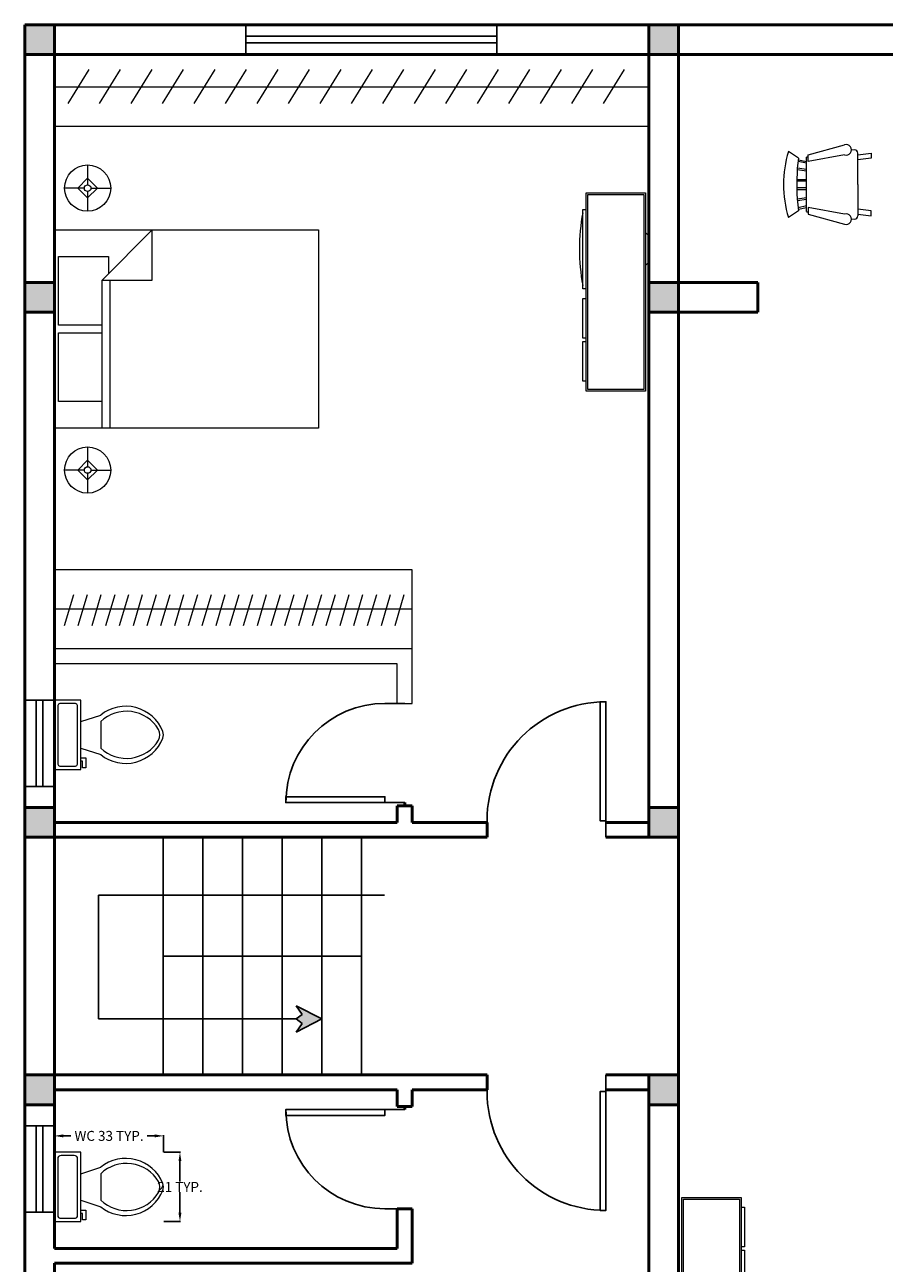
# Model space of a CAD drawing. Units: inches. Extents: x 13 to 1693, y -7 to 1519.
# Tile 2 of 10: x 116 to 377, y 360 to 735. Entities that reach past the tile are written whole.
import ezdxf

# ---------------------------------------------------------------- set-up
doc = ezdxf.new("R2010")
doc.units = ezdxf.units.IN
doc.header["$MEASUREMENT"] = 0
for name, color, linetype, lineweight in [('A-ANNO-DIMS', 2, 'Continuous', 18), ('A-DOOR', 4, 'Continuous', 25), ('A-FLOR-CASE', 5, 'Continuous', 18), ('A-FLOR-FIXT', 9, 'Continuous', 18), ('A-FLOR-STRS', 2, 'Continuous', 25), ('A-FURN', 8, 'Continuous', 18), ('A-GLAZ', 4, 'Continuous', 25), ('A-WALL', 7, 'Continuous', 50), ('A-WALL-PATT', 8, 'Continuous', 13)]:
    doc.layers.add(name, color=color, linetype=linetype, lineweight=lineweight)
doc.styles.get("Standard").update_dxf_attribs({"font": 'arial.ttf'})
doc.dimstyles.get("Standard").update_dxf_attribs({"dimtxt": 3, "dimasz": 2.68, "dimexe": 0.18, "dimexo": 0.0625, "dimgap": 0.09, "dimtad": 0, "dimtih": 1, "dimtoh": 1, "dimdec": 0, "dimzin": 0, "dimdsep": 46, "dimlunit": 3, "dimtxsty": 'Standard', "dimcen": 0.09, "dimadec": 0, "dimazin": 0, "dimtfac": 1, "dimtdec": 0, "dimtofl": 0, "dimtmove": 0, "dimatfit": 3, "dimfxl": 1, "dimtolj": 1, "dimtzin": 0, "dimarcsym": 0})

# ---------------------------------------------------------------- blocks, each defined once
blk = doc.blocks.new('*U7')
for p, q in [((0, 0), (0, -5)), ((36, 0), (36, -5))]:
    blk.add_line(p, q)
blk.add_lwpolyline([(0, 0), (0, 36), (1.75, 36), (1.75, 0)], close=True)
blk.add_arc((0, 0), 36, 0, 90)
blk = doc.blocks.new('*U8')
for p, q in [((0, 0), (0, -6)), ((30, 0), (30, -6))]:
    blk.add_line(p, q)
blk.add_lwpolyline([(0, 0), (0, 30), (1.75, 30), (1.75, 0)], close=True)
blk.add_arc((0, 0), 30, 0, 90)
blk = doc.blocks.new('Entertainment Center')
for p, q in [((-4, 0), (-5, -1)), ((4, 0), (-4, 0)), ((5, -1), (4, 0)), ((-17, -19), (-17, -1)), ((-17, -1), (43, -1)), ((-16.5, -18.5), (-16.5, -1.5)), ((-16.5, -1.5), (42.5, -1.5)), ((42.5, -1.5), (42.5, -18.5)), ((43, -1), (43, -19)), ((42.5, -18.5), (-16.5, -18.5)), ((43, -19), (-17, -19)), ((-12, -20), (-12, -19)), ((12, -20), (-12, -20)), ((12, -19), (12, -20)), ((15, -20), (15, -19)), ((27, -20), (15, -20)), ((27, -19), (27, -20)), ((28, -20), (28, -19)), ((40, -20), (28, -20)), ((40, -19), (40, -20))]:
    blk.add_line(p, q)
blk.add_arc((0, 40), 61, 259.6111, 280.3889)
blk = doc.blocks.new('Bed - Queen')
for p, q in [((0, -80.00003), (0, 0)), ((0, 0), (59.99999, 0)), ((59.99999, 0), (59.99999, -80.00003)), ((7.99999, -1.2), (28.79998, -1.2)), ((7.99999, -14.4), (7.99999, -1.2)), ((28.79998, -1.2), (28.79998, -14.4)), ((31.19999, -1.2), (51.99999, -1.2)), ((31.19999, -14.4), (31.19999, -1.2)), ((51.99999, -1.2), (51.99999, -16.4)), ((0, -14.4), (44.8, -14.4)), ((59.99999, -29.6), (44.8, -14.4)), ((44.8, -14.4), (44.8, -29.6)), ((44.8, -16.8), (0, -16.8)), ((51.99999, -16.4), (46.79936, -16.4)), ((44.8, -29.6), (59.99999, -29.6)), ((59.99999, -80.00003), (0, -80.00003))]:
    blk.add_line(p, q)
blk = doc.blocks.new('Lamp - Table')
for p, q in [((0, 7), (0, 1)), ((-1, 0), (-7, 0)), ((0, 3), (-3, 0)), ((-3, 0), (0, -3)), ((3, 0), (0, 3)), ((0, -3), (3, 0)), ((1, 0), (7, 0)), ((0, -1), (0, -7))]:
    blk.add_line(p, q)
for radius in [7, 1]:
    blk.add_circle((0, 0), radius)
blk = doc.blocks.new('Toilet - top')
for p, q in [((9.5, -6), (9.5, -2)), ((-10, -8.5), (-8, -8.5)), ((-10, -9.5), (-10, -8.5)), ((-7, -9.5), (-10, -9.5)), ((-8, -8.5), (-8, -8)), ((-7, -8), (-7, -9.5)), ((-4, -8), (-6, -14)), ((4, -8), (6, -14)), ((4, -14), (-4, -14))]:
    blk.add_line(p, q)
blk.add_lwpolyline([(10.5, -8), (10.5, 0), (-10.5, 0), (-10.5, -8)], close=True)
for points in [[(-9.5, -2), (-9.5, -6)], [(8.5, -1), (-8.5, -1)], [(-8.5, -7), (8.5, -7)]]:
    blk.add_lwpolyline(points)
for centre, radius, start, end in [((-8.62, -1.88), 0.884, 81.8699, 188.1301), ((8.62, -1.88), 0.884, 351.8699, 98.1301), ((-8.62, -6.12), 0.884, 171.8699, 278.1301), ((8.62, -6.12), 0.884, 261.8699, 8.1301), ((3.52, -21.58), 12.17, 141.4691, 247.9714), ((4.2, -21.82), 11.33, 136.3677, 238.9468), ((-3.52, -21.58), 12.17, 292.0284, 38.5307), ((-4.2, -21.82), 11.33, 301.053, 43.6321), ((0, -27.88), 4, 245.7318, 294.2682), ((0, -29), 4, 254.8605, 285.1395)]:
    blk.add_arc(centre, radius, start, end)
blk = doc.blocks.new('Chair - Rocking')
for p, q in [((-8, -4.5), (-10, -1.5)), ((8, -4.5), (10, -1.5)), ((-9, -7.5), (-12, -18.49999)), ((-7, -7.5), (-9, -7.5)), ((-9, -18.49999), (-7, -7.5)), ((-8.23428, -6.99939), (-8.3093, -7.47958)), ((-8.23041, -7), (8.23915, -7)), ((-7.5, -4.5), (-7, -7)), ((-6.5, -7), (-7.02225, -4.43)), ((-4.5, -7), (-4.96674, -4.19951)), ((-4, -7), (-4.40532, -4.16272)), ((-1.5, -4.05012), (-1.5, -7)), ((-1, -7), (-1, -4.05012)), ((1, -7), (1, -4.04655)), ((1.5, -4.05012), (1.5, -7)), ((4, -7), (4.40187, -4.18694)), ((4.5, -7), (4.96761, -4.19437)), ((6.5, -7), (7, -4.4057)), ((7.5, -4.5), (7, -7)), ((7, -7.5), (9, -7.5)), ((9, -18.49999), (7, -7.5)), ((8.31071, -7.48854), (8.23449, -7.00073)), ((9, -7.5), (12, -18.49999)), ((-10.36644, -20.64523), (-10.5, -21.49999)), ((-9, -22.49999), (-9.5, -26.49999)), ((0, -22.49999), (-9.5, -22.49999)), ((-8, -26.49999), (-7.5, -22.49999)), ((0, -22.49999), (9.5, -22.49999)), ((8, -26.49999), (7.5, -22.49999)), ((9, -22.49999), (9.5, -26.49999)), ((10.5, -21.49999), (10.3575, -20.58798)), ((-9.5, -26.49999), (-8, -26.49999)), ((9.5, -26.49999), (8, -26.49999))]:
    blk.add_line(p, q)
for centre, radius, start, end in [((0, -34.08333), 34.08333, 72.93847, 107.0615), ((0, -68.25004), 64.25, 93.92211, 97.15267), ((0, -68.25004), 64.25, 82.84733, 93.92211), ((-10.5, -18.99999), 1.58114, 161.5651, 18.43495), ((10.5, -18.99999), 1.58114, 161.5651, 18.43495), ((-9.5, -21.49999), 1, 180, 270), ((9.5, -21.49999), 1, 270, 0)]:
    blk.add_arc(centre, radius, start, end)
blk = doc.blocks.new('WIN-76')
for p, q in [((0, 9), (0, 0)), ((76.02, 9), (76.02, 0)), ((0, 5.5), (76.02, 5.5)), ((0, 3.5), (76.02, 3.5))]:
    blk.add_line(p, q)
blk = doc.blocks.new('WIN-26')
for p, q in [((9, 26.11), (0, 26.11)), ((3.5, 26.11), (3.5, 0)), ((5.5, 26.11), (5.5, 0)), ((9, 0), (0, 0))]:
    blk.add_line(p, q)
blk = doc.blocks.new('*D64')
at = {"layer": 'A-ANNO-DIMS', "color": 0, "lineweight": -2, "transparency": 16777216}
for p, q in [((125.45, 393.82), (125.45, 398.89)), ((128.13, 398.71), (130.45, 398.71)), ((155.82, 398.71), (153.5, 398.71)), ((158.5, 393.82), (158.5, 398.89))]:
    blk.add_line(p, q, dxfattribs=at)
at = {"layer": 'A-ANNO-DIMS', "color": 0, "transparency": 16777216}
for points in [[(128.13, 399.16), (128.13, 398.26), (125.45, 398.71)], [(155.82, 399.16), (155.82, 398.26), (158.5, 398.71)]]:
    blk.add_solid(points, dxfattribs=at)
at = {"layer": 'Defpoints', "color": 0, "transparency": 16777216}
for p in [(125.45, 398.71), (125.45, 393.75), (158.5, 393.75)]:
    blk.add_point(p, dxfattribs=at)
at = {"layer": 'A-ANNO-DIMS', "color": 0, "transparency": 16777216, "insert": (141.98, 398.71), "char_height": 3, "attachment_point": 5}
blk.add_mtext('\\A1;WC 33 TYP.', dxfattribs=at)
blk = doc.blocks.new('*D65')
at = {"layer": 'A-ANNO-DIMS', "color": 0, "lineweight": -2, "transparency": 16777216}
for p, q in [((158.56, 393.75), (163.64, 393.75)), ((163.46, 391.07), (163.46, 384.85)), ((163.46, 375.43), (163.46, 381.66)), ((158.56, 372.75), (163.64, 372.75))]:
    blk.add_line(p, q, dxfattribs=at)
at = {"layer": 'A-ANNO-DIMS', "color": 0, "transparency": 16777216}
for points in [[(163.01, 391.07), (163.9, 391.07), (163.46, 393.75)], [(163.01, 375.43), (163.9, 375.43), (163.46, 372.75)]]:
    blk.add_solid(points, dxfattribs=at)
at = {"layer": 'Defpoints', "color": 0, "transparency": 16777216}
for p in [(158.5, 393.75), (163.46, 393.75), (158.5, 372.75)]:
    blk.add_point(p, dxfattribs=at)
at = {"layer": 'A-ANNO-DIMS', "color": 0, "transparency": 16777216, "insert": (163.46, 383.25), "char_height": 3, "attachment_point": 5}
blk.add_mtext('\\A1;21 TYP.', dxfattribs=at)

msp = doc.modelspace()

# ---------------------------------------------------------------- hatches: boundary and pattern name
at = {"layer": 'A-WALL-PATT'}
h = msp.add_hatch(color=256, dxfattribs=at)
h.dxf.hatch_style = 1
h.paths.add_polyline_path([(125.45, 735.15), (116.45, 735.15), (116.45, 726.15), (125.45, 726.15)])
h.paths.add_polyline_path([(125.45, 657.15), (116.45, 657.15), (116.45, 648.15), (125.45, 648.15)])
h.paths.add_polyline_path([(125.45, 498.15), (116.45, 498.15), (116.45, 489.15), (125.45, 489.15)])
h.paths.add_polyline_path([(125.45, 417.15), (116.45, 417.15), (116.45, 408.15), (125.45, 408.15)])
h.paths.add_polyline_path([(125.45, 177.15), (116.45, 177.15), (116.45, 168.15), (125.45, 168.15)])
h.paths.add_polyline_path([(314.45, 177.15), (305.45, 177.15), (305.45, 168.15), (314.45, 168.15)])
h.paths.add_polyline_path([(314.45, 417.15), (305.45, 417.15), (305.45, 408.15), (314.45, 408.15)])
h.paths.add_polyline_path([(314.45, 498.15), (305.45, 498.15), (305.45, 489.15), (314.45, 489.15)])
h.paths.add_polyline_path([(314.45, 657.15), (305.45, 657.15), (305.45, 648.15), (314.45, 648.15)])
h.paths.add_polyline_path([(314.45, 735.15), (305.45, 735.15), (305.45, 726.15), (314.45, 726.15)])
h = msp.add_hatch(color=256, dxfattribs=at)
h.dxf.hatch_style = 1
h.paths.add_polyline_path([(198.64, 438.07), (200.46, 435.46), (198.61, 434.11), (200.46, 432.76), (198.64, 430.15), (206.42, 434.11)])

# ---------------------------------------------------------------- linework, layer by layer
at = {"layer": 'A-FLOR-CASE'}
for p, q in [((135.81, 721.58), (129.45, 711.36)), ((145.35, 721.58), (138.99, 711.36)), ((154.89, 721.58), (148.53, 711.36)), ((164.43, 721.58), (158.07, 711.36)), ((173.97, 721.58), (167.61, 711.36)), ((183.51, 721.58), (177.15, 711.36)), ((193.05, 721.58), (186.69, 711.36)), ((202.59, 721.58), (196.23, 711.36)), ((212.13, 721.58), (205.77, 711.36)), ((221.67, 721.58), (215.31, 711.36)), ((231.21, 721.58), (224.85, 711.36)), ((240.75, 721.58), (234.39, 711.36)), ((250.29, 721.58), (243.93, 711.36)), ((259.82, 721.58), (253.46, 711.36)), ((269.36, 721.58), (263, 711.36)), ((278.9, 721.58), (272.54, 711.36)), ((288.44, 721.58), (282.08, 711.36)), ((297.98, 721.58), (291.62, 711.36)), ((125.45, 716.33), (305.45, 716.33)), ((125.45, 704.45), (305.45, 704.45)), ((233.77, 570.15), (125.45, 570.15)), ((233.77, 546.15), (233.77, 570.15)), ((131.17, 562.5), (128.39, 553.12)), ((135.35, 562.5), (132.56, 553.12)), ((139.52, 562.5), (136.74, 553.12)), ((143.69, 562.5), (140.91, 553.12)), ((147.86, 562.5), (145.08, 553.12)), ((152.04, 562.5), (149.25, 553.12)), ((156.21, 562.5), (153.43, 553.12)), ((160.38, 562.5), (157.6, 553.12)), ((164.55, 562.5), (161.77, 553.12)), ((168.72, 562.5), (165.94, 553.12)), ((172.9, 562.5), (170.12, 553.12)), ((177.07, 562.5), (174.29, 553.12)), ((181.24, 562.5), (178.46, 553.12)), ((185.41, 562.5), (182.63, 553.12)), ((189.59, 562.5), (186.81, 553.12)), ((193.76, 562.5), (190.98, 553.12)), ((197.93, 562.5), (195.15, 553.12)), ((202.1, 562.5), (199.32, 553.12)), ((206.28, 562.5), (203.49, 553.12)), ((210.45, 562.5), (207.67, 553.12)), ((214.62, 562.5), (211.84, 553.12)), ((218.79, 562.5), (216.01, 553.12)), ((222.97, 562.5), (220.18, 553.12)), ((227.14, 562.5), (224.36, 553.12)), ((231.31, 562.5), (228.53, 553.12)), ((233.77, 558.15), (125.45, 558.15)), ((233.77, 546.15), (125.45, 546.15)), ((233.77, 529.65), (233.77, 546.15)), ((229.27, 541.65), (125.45, 541.65)), ((229.27, 529.65), (229.27, 541.65)), ((229.27, 529.65), (233.77, 529.65))]:
    msp.add_line(p, q, dxfattribs=at)
at = {"layer": 'A-FLOR-STRS'}
for p, q in [((158.42, 489.15), (158.42, 417.15)), ((170.42, 489.15), (170.42, 417.15)), ((182.42, 489.15), (182.42, 417.15)), ((194.42, 489.15), (194.42, 417.15)), ((206.42, 489.15), (206.42, 417.15)), ((218.42, 489.15), (218.42, 417.15)), ((225.37, 471.55), (138.82, 471.55)), ((138.82, 471.55), (138.82, 434.11)), ((158.42, 453.15), (218.42, 453.15)), ((200.46, 435.46), (198.61, 434.11)), ((206.42, 434.11), (198.64, 438.07)), ((198.64, 438.07), (200.46, 435.46)), ((138.82, 434.11), (198.61, 434.11)), ((200.46, 432.76), (198.61, 434.11)), ((206.42, 434.11), (198.64, 430.15)), ((198.64, 430.15), (200.46, 432.76))]:
    msp.add_line(p, q, dxfattribs=at)
at = {"layer": 'A-WALL'}
for p, q in [((116.45, 168.15), (116.45, 735.15)), ((683.45, 735.15), (116.45, 735.15)), ((125.45, 364.65), (125.45, 735.15)), ((305.45, 735.15), (305.45, 489.15)), ((314.45, 735.15), (314.45, 489.15)), ((485.45, 726.15), (116.45, 726.15)), ((125.45, 657.15), (116.45, 657.15)), ((338.45, 657.15), (305.45, 657.15)), ((338.45, 648.15), (338.45, 657.15)), ((125.45, 648.15), (116.45, 648.15)), ((338.45, 648.15), (305.45, 648.15)), ((231.52, 498.65), (231.52, 499.65)), ((229.27, 493.65), (229.27, 498.65)), ((233.77, 498.65), (229.27, 498.65)), ((233.77, 493.65), (233.77, 498.65)), ((233.77, 493.65), (233.77, 498.65)), ((229.27, 493.65), (125.45, 493.65)), ((256.45, 493.65), (233.77, 493.65)), ((256.45, 493.65), (256.45, 489.15)), ((305.45, 493.65), (292.45, 493.65)), ((256.45, 489.15), (116.45, 489.15)), ((293.45, 489.15), (292.45, 489.15)), ((314.45, 489.15), (293.45, 489.15)), ((314.45, 489.15), (314.45, 417.15)), ((256.45, 417.15), (116.45, 417.15)), ((256.45, 412.65), (256.45, 417.15)), ((293.45, 417.15), (292.45, 417.15)), ((314.45, 417.15), (293.45, 417.15)), ((305.45, 417.15), (305.45, 168.15)), ((314.45, 417.15), (314.45, 222.15)), ((229.27, 412.65), (125.45, 412.65)), ((229.27, 412.65), (229.27, 407.65)), ((256.45, 412.65), (233.77, 412.65)), ((233.77, 412.65), (233.77, 407.65)), ((233.77, 412.65), (233.77, 407.65)), ((305.45, 412.65), (292.45, 412.65)), ((233.77, 407.65), (229.27, 407.65)), ((231.52, 407.65), (231.52, 406.65)), ((229.27, 376.65), (229.27, 364.65)), ((229.27, 376.65), (233.77, 376.65)), ((233.77, 376.65), (233.77, 360.15)), ((229.27, 364.65), (125.45, 364.65)), ((125.45, 168.15), (125.45, 360.15)), ((233.77, 360.15), (125.45, 360.15))]:
    msp.add_line(p, q, dxfattribs=at)
for points in [[(116.45, 489.15), (125.45, 489.15), (125.45, 498.15), (116.45, 498.15)], [(305.45, 489.15), (314.45, 489.15), (314.45, 498.15), (305.45, 498.15)], [(116.45, 408.15), (125.45, 408.15), (125.45, 417.15), (116.45, 417.15)], [(305.45, 408.15), (314.45, 408.15), (314.45, 417.15), (305.45, 417.15)]]:
    msp.add_lwpolyline(points, close=True, dxfattribs=at)

# ---------------------------------------------------------------- block references
at = {"layer": 'A-DOOR'}
for name, p, rotation in [('*U8', (225.52, 499.65), 90), ('*U7', (292.45, 412.15), 180)]:
    msp.add_blockref(name, p, dxfattribs=dict(at, rotation=rotation))
at = {"layer": 'A-DOOR', "xscale": -1}
msp.add_blockref('*U7', (292.45, 494.15), dxfattribs=at)
at = {"layer": 'A-DOOR', "xscale": -1, "rotation": 90}
msp.add_blockref('*U8', (225.52, 406.65), dxfattribs=at)
at = {"layer": 'A-FLOR-FIXT', "rotation": 89.99999999999999}
for p in [(125.45, 520.15), (125.45, 383.25)]:
    msp.add_blockref('Toilet - top', p, dxfattribs=at)
at = {"layer": 'A-FURN'}
for name, p, rotation in [('Chair - Rocking', (346.25, 686.79), 90), ('Entertainment Center', (305.45, 667.24), 270), ('Bed - Queen', (125.45, 613.03), 90), ('Entertainment Center', (314.45, 337.08), 90)]:
    msp.add_blockref(name, p, dxfattribs=dict(at, rotation=rotation))
for p in [(135.5, 685.71), (135.5, 600.33)]:
    msp.add_blockref('Lamp - Table', p, dxfattribs=at)
at = {"layer": 'A-GLAZ', "rotation": 180}
for name, p in [('WIN-76', (259.41, 735.15)), ('WIN-26', (125.45, 530.65))]:
    msp.add_blockref(name, p, dxfattribs=at)
at = {"layer": 'A-GLAZ'}
msp.add_blockref('WIN-26', (116.45, 375.65), dxfattribs=at)

# ---------------------------------------------------------------- dimensions: what is measured, and where the dimension line sits
at = {"layer": 'A-ANNO-DIMS'}
for base, p1, p2, angle, text, picture, middle in [((125.45, 398.71), (158.5, 393.75), (125.45, 393.75), 180, 'WC <> TYP.', '*D64', (141.98, 398.71)), ((163.46, 393.75), (158.5, 372.75), (158.5, 393.75), 90, '<> TYP.', '*D65', (163.46, 383.25))]:
    dim = msp.add_linear_dim(base=base, p1=p1, p2=p2, angle=angle, text=text, dimstyle='Standard', override={"dimdec": 0, "dimlfac": 1, "dimrnd": 0, "dimzin": 0, "dimdsep": 46, "dimlunit": 2}, dxfattribs=at)
    dim.commit()
    dim.dimension.update_dxf_attribs({"geometry": picture, "text_midpoint": middle})

doc.saveas('drawing.dxf')
